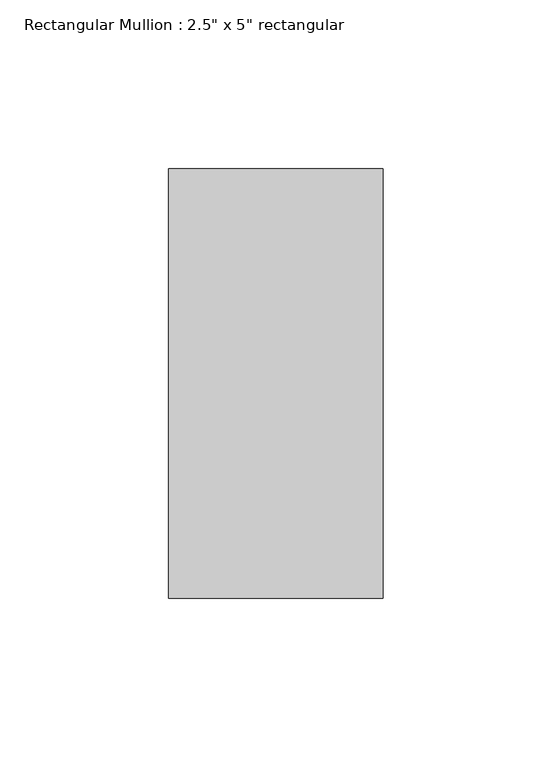
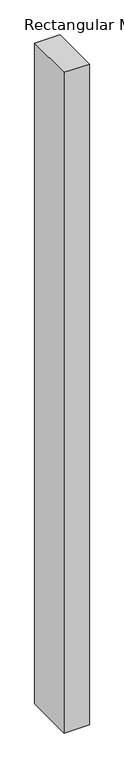
"""IFC4 building model written with IfcOpenShell, lengths in millimetres: member geometry."""

from ifc_helpers import new_model, si_unit, frame, origin, place, context, project, spatial, polyline, outline, extrude, source, transform, mapped, element, save


def member_2bb4249f(model_context):
    return source(origin(), model_context, "Body", "SweptSolid", [
        extrude(outline(polyline([(0.0, 63.5), (0.0, -63.5), (-63.5, -63.5), (-63.5, 63.5), (0.0, 63.5)])), frame((0.0, 0.0, -1748.0218004), z_axis=(0.0, 0.0, 1.0), x_axis=(1.0, 0.0, 0.0)), (0.0, 0.0, 1.0), 1748.0218004),
    ])


if __name__ == "__main__":
    model = new_model("IFC4")
    model_context = context("Model", 3, world=origin())
    ifc_project = project(units=[si_unit("LENGTHUNIT", "METRE", prefix="MILLI")], contexts=[model_context])
    site = spatial("IfcSite", under=ifc_project)
    building = spatial("IfcBuilding", under=site)
    placement = place(None, origin())
    member_shape = member_2bb4249f(model_context)
    element("IfcMember", 1, ObjectType="Rectangular Mullion : 2.5\" x 5\" rectangular", at=placement, inside=building, context=model_context, shape_type="MappedRepresentation", body=[
        mapped(member_shape, transform((0.0, 0.0, 0.0), x_axis=(1.0, 0.0, 0.0), y_axis=(0.0, 1.0, 0.0), z_axis=(0.0, 0.0, 1.0))),
    ])
    save(model, "model.ifc")

# Revit data of these elements
# Type "Rectangular Mullion : 2.5\" x 5\" rectangular"
#   built-in parameter 1007304 = 0.416667 (stored number, unit not read)
#   built-in parameter 1007301 = 0.104167 (stored number, unit not read)
#   built-in parameter 1007300 = 0.104167 (stored number, unit not read)
# Element 1 (IfcMember, "Rectangular Mullion : 2.5\" x 5\" rectangular")
#   Materials on its faces: "Aluminum"
# Materials
#   "Aluminum": class "Metal", colour RGB 247 247 247, transparency 0, Description = "Aluminum 6061", Cost = 0
